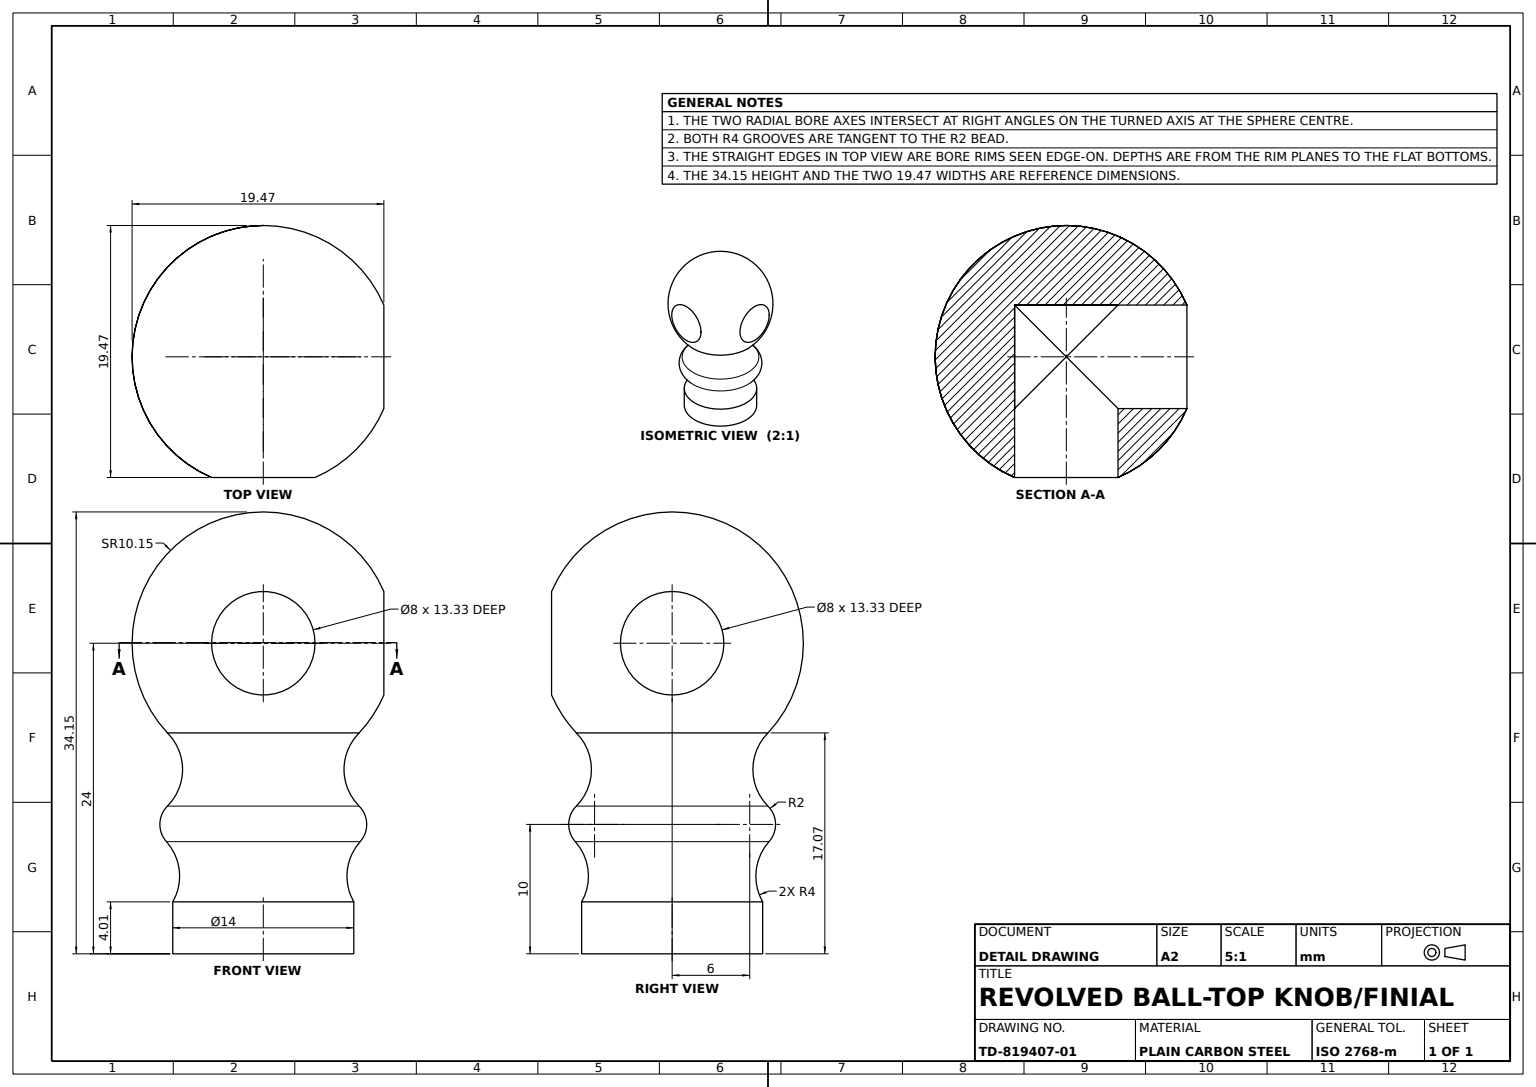
from build123d import *

# Parameters (mm, degrees)
SIDE_CUT_A_8_DEPTH      = 4
SIDE_CUT_A_8_DEPTH_BACK = 14
SIDE_CUT_A_8_SKETCH_R   = 4
SIDE_CUT_B_8_DEPTH      = 4
SIDE_CUT_B_8_DEPTH_BACK = 14
SIDE_CUT_B_8_SKETCH_R   = 4


with BuildPart() as part:
    # Knob Profile Sketch → Knob Body Revolve (revolve)
    with BuildSketch(Plane.XY, mode=Mode.PRIVATE) as knob_body_revolve_sk:
        with BuildLine():
            Line((0, 24), (0, 0))
            Line((0, 0), (7, 0))
            Line((7, 0), (7, 4.013980889))
            ThreePointArc((7, 4.013980889), (6.494199283, 6.419547181), (7.490711985, 8.666666667))
            ThreePointArc((7.490711985, 8.666666667), (7.999225249, 10.055663319), (7.414213562, 11.414213562))
            ThreePointArc((7.414213562, 11.414213562), (6.243817658, 14.14561297), (7.28036451, 16.930561789))
            ThreePointArc((7.28036451, 16.930561789), (7.34643685, 17.001626612), (7.414213562, 17.071067812))
            ThreePointArc((7.414213562, 17.071067812), (9.308465087, 28.041428182), (0, 34.147938905))
            Line((0, 34.147938905), (0, 24))
        make_face()
    revolve(knob_body_revolve_sk.sketch.rotate(Axis((0, 0, 0), (0, 1, 0)), 90), axis=Axis((0, 0, 0), (0, 1, 0)))

    # Side Cut A Ø8 Sketch → Side Cut A Ø8 (cut, two sides: drawn at the far end of the back side and taken through both)
    with BuildSketch(Plane.XY.offset(-SIDE_CUT_A_8_DEPTH_BACK)):
        with Locations((0, 24)):
            Circle(SIDE_CUT_A_8_SKETCH_R)
    extrude(amount=SIDE_CUT_A_8_DEPTH + SIDE_CUT_A_8_DEPTH_BACK, mode=Mode.SUBTRACT)

    # Side Cut B Ø8 Sketch → Side Cut B Ø8 (cut, two sides: drawn at the far end of the back side and taken through both)
    with BuildSketch(Plane(origin=(0, 0, 0), x_dir=(0, 0, -1), z_dir=(1, 0, 0)).offset(-SIDE_CUT_B_8_DEPTH_BACK)):
        with Locations(Location((0, 24, 0), (0, 0, 180))):
            Circle(SIDE_CUT_B_8_SKETCH_R)
    extrude(amount=SIDE_CUT_B_8_DEPTH + SIDE_CUT_B_8_DEPTH_BACK, mode=Mode.SUBTRACT)


solid = part.part
